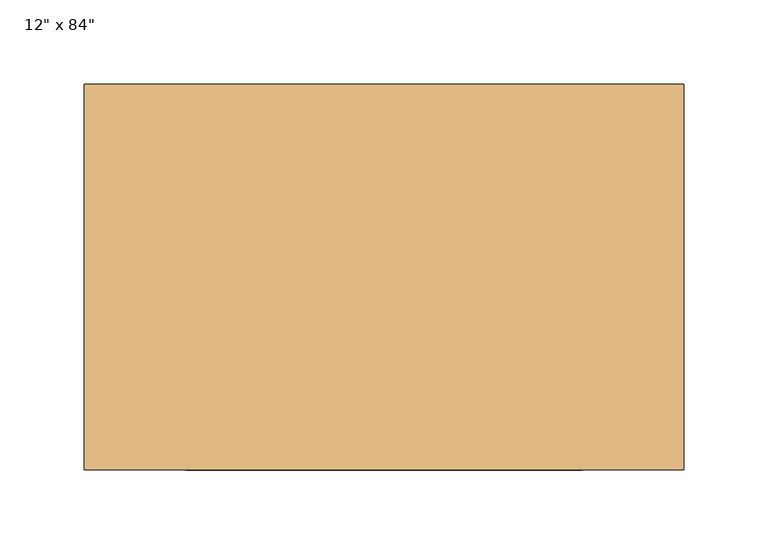
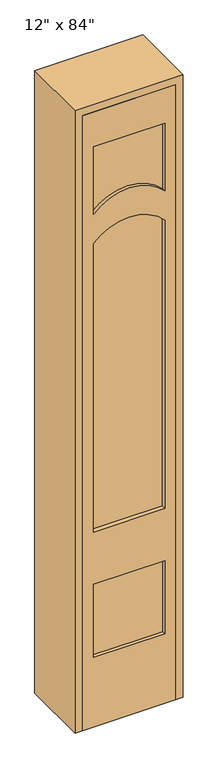
"""IFC4 building model written with IfcOpenShell, lengths in millimetres: door geometry."""

from ifc_helpers import new_model, si_unit, point, frame, frame_2d, origin, place, context, project, spatial, polyline, circle_curve, trimmed, segment, composite_curve, outline, extrude, source, transform, mapped, element, save


def door_302e125b(model_context):
    return source(origin(), model_context, "Body", "SweptSolid", [
        extrude(outline(polyline([(117.475, -87.8416667), (117.475, -99.4833333), (-117.475, -99.4833333), (-117.475, -87.8416667), (117.475, -87.8416667)])), frame((0.0, 0.0, 241.3), z_axis=(0.0, 0.0, 1.0), x_axis=(1.0, 0.0, 0.0)), (0.0, 0.0, 1.0), 254.0),
        extrude(outline(composite_curve([segment(polyline([(1778.0, 117.475), (2012.95, 117.475), (2012.95, -117.475), (1778.0, -117.475)]), True, "CONTINUOUS"), segment(trimmed(circle_curve(frame_2d((1667.5695312, 0.0)), 161.2304687), [point((1778.0, -117.475))], [point((1778.0, 117.475))], True, "CARTESIAN"), True, "CONTINUOUS")], self_intersect=False)), frame((0.0, -99.4833333, 0.0), z_axis=(0.0, 1.0, 0.0), x_axis=(0.0, 0.0, 1.0)), (0.0, 0.0, 1.0), 11.6416667),
        extrude(outline(polyline([(2133.6, -152.4), (0.0, -152.4), (0.0, 152.4), (2133.6, 152.4), (2133.6, -152.4)]), holes=[composite_curve([segment(polyline([(676.275, -117.475), (1676.4, -117.475)]), True, "CONTINUOUS"), segment(trimmed(circle_curve(frame_2d((1565.9695312, 0.0)), 161.2304688), [point((1676.4, -117.475))], [point((1676.4, 117.475))], True, "CARTESIAN"), True, "CONTINUOUS"), segment(polyline([(1676.4, 117.475), (676.275, 117.475), (676.275, -117.475)]), True, "CONTINUOUS")], self_intersect=False), polyline([(495.3, -117.475), (495.3, 117.475), (241.3, 117.475), (241.3, -117.475), (495.3, -117.475)]), composite_curve([segment(polyline([(2012.95, -117.475), (2012.95, 117.475), (1778.0, 117.475)]), True, "CONTINUOUS"), segment(trimmed(circle_curve(frame_2d((1667.5695312, 0.0)), 161.2304687), [point((1778.0, 117.475))], [point((1778.0, -117.475))], False, "CARTESIAN"), True, "CONTINUOUS"), segment(polyline([(1778.0, -117.475), (2012.95, -117.475)]), True, "CONTINUOUS")], self_intersect=False)]), frame((0.0, -111.125, 0.0), z_axis=(0.0, 1.0, 0.0), x_axis=(0.0, 0.0, 1.0)), (0.0, 0.0, 1.0), 34.925),
        extrude(outline(polyline([(0.0, 177.8), (2159.0, 177.8), (2159.0, -177.8), (0.0, -177.8), (0.0, -152.4), (2133.6, -152.4), (2133.6, 152.4), (0.0, 152.4), (0.0, 177.8)])), frame((0.0, -111.125, 0.0), z_axis=(0.0, 1.0, 0.0), x_axis=(0.0, 0.0, 1.0)), (0.0, 0.0, 1.0), 228.6),
        extrude(outline(composite_curve([segment(polyline([(676.275, -117.475), (676.275, 117.475), (1676.4, 117.475)]), True, "CONTINUOUS"), segment(trimmed(circle_curve(frame_2d((1565.9695312, 0.0)), 161.2304688), [point((1676.4, 117.475))], [point((1676.4, -117.475))], False, "CARTESIAN"), True, "CONTINUOUS"), segment(polyline([(1676.4, -117.475), (676.275, -117.475)]), True, "CONTINUOUS")], self_intersect=False)), frame((0.0, -97.155, 0.0), z_axis=(0.0, 1.0, 0.0), x_axis=(0.0, 0.0, 1.0)), (0.0, 0.0, 1.0), 6.985),
    ])


if __name__ == "__main__":
    model = new_model("IFC4")
    model_context = context("Model", 3, world=origin())
    ifc_project = project(units=[si_unit("LENGTHUNIT", "METRE", prefix="MILLI")], contexts=[model_context])
    site = spatial("IfcSite", under=ifc_project)
    building = spatial("IfcBuilding", under=site)
    placement = place(None, origin())
    door_shape = door_302e125b(model_context)
    element("IfcDoor", 1, ObjectType="12\" x 84\"", at=placement, inside=building, context=model_context, shape_type="MappedRepresentation", body=[
        mapped(door_shape, transform((0.0, 0.0, 0.0), x_axis=(1.0, 0.0, 0.0), y_axis=(0.0, 1.0, 0.0), z_axis=(0.0, 0.0, 1.0))),
    ])
    save(model, "model.ifc")

# Revit data of these elements
# Type "12\" x 84\""
#   Type Mark = "9"
#   Assembly Code = "B2030100"
#   Analytic Construction = "French door, wood frame with single glass"
#   Radius = 0' - 6 89/256"
#   Lock Rail = 0' - 7 1/8"
#   Thickness = 0' - 1 3/8"
#   Thermal Resistance (R) = 1.0696 (h·ft²·°F)/BTU
#   Stiles = 0' - 1 3/8"
#   Rough Width = 1' - 2"
#   Rough Height = 7' - 1"
#   Height = 7' - 0"
#   Width = 1' - 0"
#   Heat Transfer Coefficient (U) = 0.9350 BTU/(h·ft²·°F)
#   Door Offset [instance default] = 0' - 0"
#   Bottom Rail = 0' - 9 1/2"
#   Function = 1
#   Trim Material = Cherry
#   Panel Material = Cherry
#   Glazing = Glass
#   Frame Material = Cherry
#   Visual Light Transmittance = 0
#   Solar Heat Gain Coefficient = 0
#   Wall Closure = (empty or 0)
#   Construction Type = (empty or 0)
# Element 1 (IfcDoor, "12\" x 84\"")
#   Materials on its faces: "Cherry", "Glass"
# Materials
#   "Cherry": class "Wood", colour RGB 226 177 128, transparency 0, Description = "Prunus Serotina", Cost = 0
#   "Glass": class "Glass", colour RGB 0 128 192, transparency 0.75, Description = "Soda Lime Glass", Cost = 0
